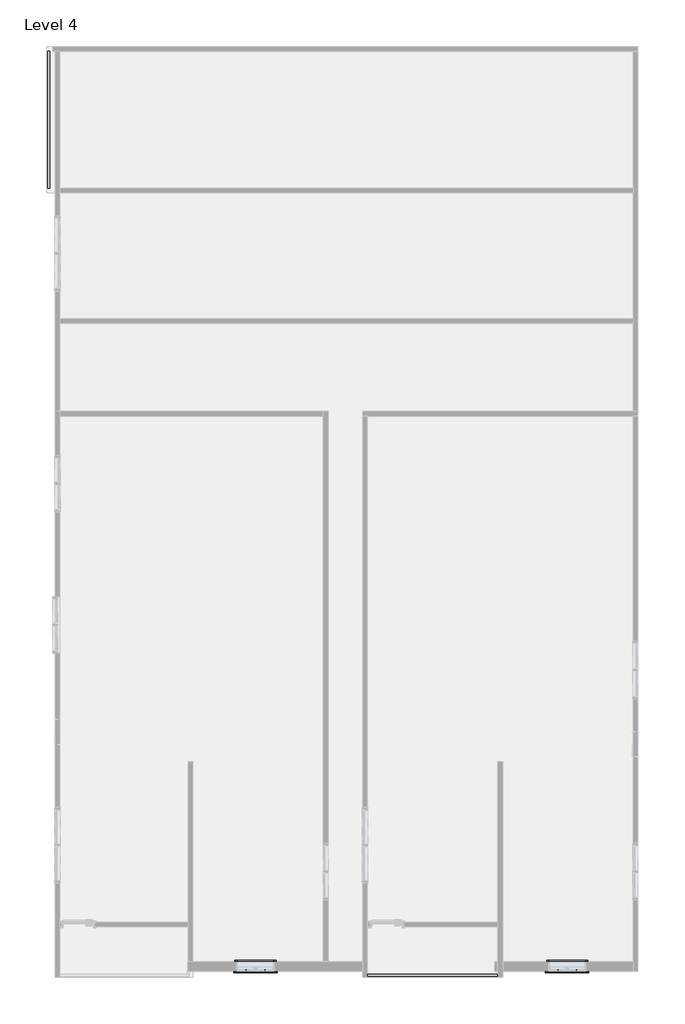
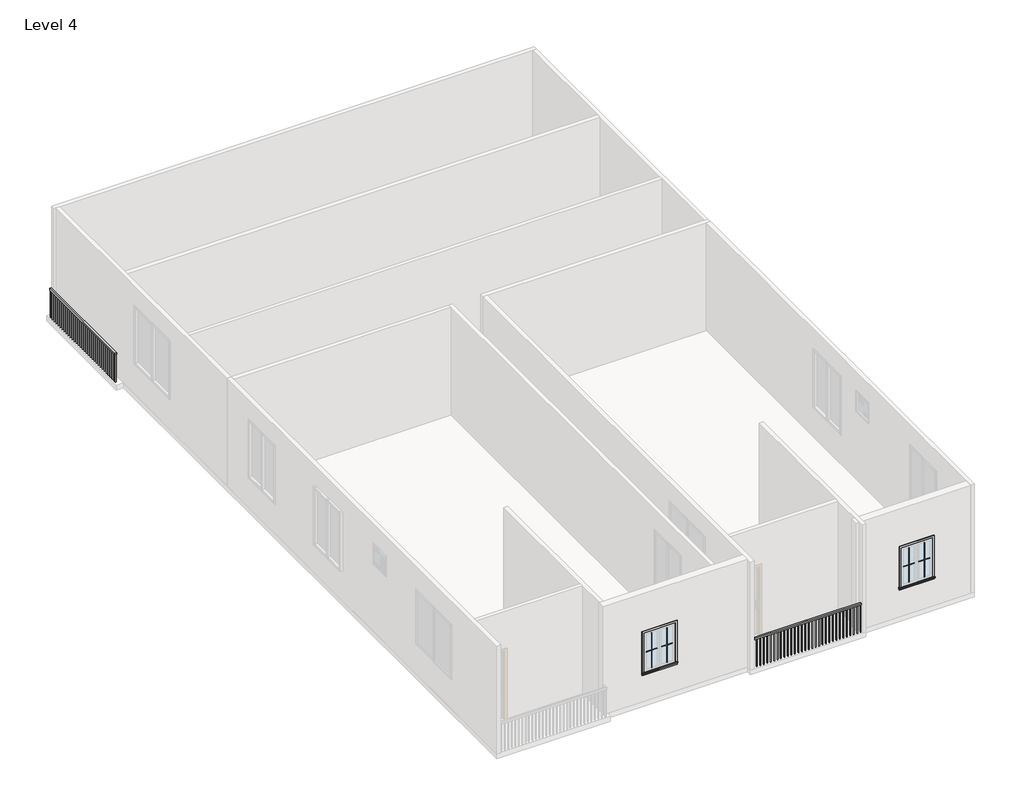
# One storey, part 3 of 3: 8 proxies, 3 railings.
"""IFC4 building model written with IfcOpenShell, lengths in millimetres."""

from ifc_helpers import new_model, si_unit, frame, origin, place, context, project, spatial, polyline, outline, extrude, transform, mapped, element, save
from components import muntin_pattern_2x2_muntin_pattern_2x2_1acec82f, muntin_pattern_2x2_muntin_pattern_2x2_43d02eee, trim_window_exterior_flat_with_sill_e4b28ec3, trim_window_interior_flat_picture_frame_39ff4276

model = new_model("IFC4")

# Units and contexts
model_context = context("Model", 3, world=origin())
ifc_project = project(units=[si_unit("LENGTHUNIT", "METRE", prefix="MILLI")], contexts=[model_context])

# Site, building, storey
site = spatial("IfcSite", under=ifc_project)
building = spatial("IfcBuilding", under=site)
storey = spatial("IfcBuildingStorey", under=building, Name="Level 4", Elevation=10058.4)

# Proxies
placement = place(None, origin())
muntin_pattern_2x2_muntin_pattern_2x2_shape = muntin_pattern_2x2_muntin_pattern_2x2_1acec82f(model_context)
element("IfcBuildingElementProxy", 1, Name="Muntin Pattern_2x2 : Muntin Pattern_2x2", ObjectType="Muntin Pattern_2x2 : Muntin Pattern_2x2", at=placement, inside=storey, context=model_context, shape_type="MappedRepresentation", body=[
    mapped(muntin_pattern_2x2_muntin_pattern_2x2_shape, transform((-3129.6612038, -10576.3529557, 11042.65), x_axis=(-1.0, 0.0, 0.0), y_axis=(0.0, -1.0, 0.0), z_axis=(0.0, 0.0, 1.0))),
])
element("IfcBuildingElementProxy", 2, Name="Muntin Pattern_2x2 : Muntin Pattern_2x2", ObjectType="Muntin Pattern_2x2 : Muntin Pattern_2x2", at=placement, inside=storey, context=model_context, shape_type="MappedRepresentation", body=[
    mapped(muntin_pattern_2x2_muntin_pattern_2x2_shape, transform((4424.1833786, -10576.3529557, 11042.65), x_axis=(-1.0, 0.0, 0.0), y_axis=(0.0, -1.0, 0.0), z_axis=(0.0, 0.0, 1.0))),
])
muntin_pattern_2x2_muntin_pattern_2x2_2_shape = muntin_pattern_2x2_muntin_pattern_2x2_43d02eee(model_context)
element("IfcBuildingElementProxy", 3, Name="Muntin Pattern_2x2 : Muntin Pattern_2x2", ObjectType="Muntin Pattern_2x2 : Muntin Pattern_2x2", at=placement, inside=storey, context=model_context, shape_type="MappedRepresentation", body=[
    mapped(muntin_pattern_2x2_muntin_pattern_2x2_2_shape, transform((-3583.6862038, -10576.3529557, 11042.65), x_axis=(1.0, 0.0, 0.0), y_axis=(0.0, 1.0, 0.0), z_axis=(0.0, 0.0, 1.0))),
])
element("IfcBuildingElementProxy", 4, Name="Muntin Pattern_2x2 : Muntin Pattern_2x2", ObjectType="Muntin Pattern_2x2 : Muntin Pattern_2x2", at=placement, inside=storey, context=model_context, shape_type="MappedRepresentation", body=[
    mapped(muntin_pattern_2x2_muntin_pattern_2x2_2_shape, transform((3970.1583786, -10576.3529557, 11042.65), x_axis=(1.0, 0.0, 0.0), y_axis=(0.0, 1.0, 0.0), z_axis=(0.0, 0.0, 1.0))),
])
trim_window_exterior_flat_with_sill_shape = trim_window_exterior_flat_with_sill_e4b28ec3(model_context)
element("IfcBuildingElementProxy", 5, Name="Trim-Window-Exterior-Flat : with Sill", ObjectType="Trim-Window-Exterior-Flat : with Sill", at=placement, inside=storey, context=model_context, shape_type="MappedRepresentation", body=[
    mapped(trim_window_exterior_flat_with_sill_shape, transform((-3356.6737038, -10585.8779557, 12192.0), x_axis=(1.0, 0.0, 0.0), y_axis=(0.0, 0.0, 1.0), z_axis=(0.0, -1.0, 0.0))),
])
element("IfcBuildingElementProxy", 6, Name="Trim-Window-Exterior-Flat : with Sill", ObjectType="Trim-Window-Exterior-Flat : with Sill", at=placement, inside=storey, context=model_context, shape_type="MappedRepresentation", body=[
    mapped(trim_window_exterior_flat_with_sill_shape, transform((4197.1708786, -10585.8779557, 12192.0), x_axis=(1.0, 0.0, 0.0), y_axis=(0.0, 0.0, 1.0), z_axis=(0.0, -1.0, 0.0))),
])
trim_window_interior_flat_picture_frame_shape = trim_window_interior_flat_picture_frame_39ff4276(model_context)
element("IfcBuildingElementProxy", 7, Name="Trim-Window-Interior-Flat : Picture Frame", ObjectType="Trim-Window-Interior-Flat : Picture Frame", at=placement, inside=storey, context=model_context, shape_type="MappedRepresentation", body=[
    mapped(trim_window_interior_flat_picture_frame_shape, transform((-3356.6737038, -10357.2779557, 12192.0), x_axis=(-1.0, 0.0, 0.0), y_axis=(0.0, 0.0, 1.0), z_axis=(0.0, 1.0, 0.0))),
])
element("IfcBuildingElementProxy", 8, Name="Trim-Window-Interior-Flat : Picture Frame", ObjectType="Trim-Window-Interior-Flat : Picture Frame", at=placement, inside=storey, context=model_context, shape_type="MappedRepresentation", body=[
    mapped(trim_window_interior_flat_picture_frame_shape, transform((4197.1708786, -10357.2779557, 12192.0), x_axis=(-1.0, 0.0, 0.0), y_axis=(0.0, 0.0, 1.0), z_axis=(0.0, 1.0, 0.0))),
])

# Railings
element("IfcRailing", 9, ObjectType="Handrail - Rectangular", at=placement, inside=storey, context=model_context, shape_type="SweptSolid", body=[
    extrude(outline(polyline([(-648.5431282, -10709.8005933), (-648.5431282, -10659.0005933), (2515.990751, -10659.0005933), (2515.990751, -10709.8005933), (-648.5431282, -10709.8005933)])), frame((0.0, 0.0, 10922.0), z_axis=(0.0, 0.0, 1.0), x_axis=(1.0, 0.0, 0.0)), (0.0, 0.0, 1.0), 50.8),
    extrude(outline(polyline([(2491.5318718, -10693.9255933), (2491.5318718, -10674.8755933), (2510.5818718, -10674.8755933), (2510.5818718, -10693.9255933), (2491.5318718, -10693.9255933)])), frame((0.0, 0.0, 10058.4), z_axis=(0.0, 0.0, 1.0), x_axis=(1.0, 0.0, 0.0)), (0.0, 0.0, 1.0), 863.6),
    extrude(outline(polyline([(2389.9318718, -10693.9255933), (2389.9318718, -10674.8755933), (2408.9818718, -10674.8755933), (2408.9818718, -10693.9255933), (2389.9318718, -10693.9255933)])), frame((0.0, 0.0, 10058.4), z_axis=(0.0, 0.0, 1.0), x_axis=(1.0, 0.0, 0.0)), (0.0, 0.0, 1.0), 863.6),
    extrude(outline(polyline([(2288.3318718, -10693.9255933), (2288.3318718, -10674.8755933), (2307.3818718, -10674.8755933), (2307.3818718, -10693.9255933), (2288.3318718, -10693.9255933)])), frame((0.0, 0.0, 10058.4), z_axis=(0.0, 0.0, 1.0), x_axis=(1.0, 0.0, 0.0)), (0.0, 0.0, 1.0), 863.6),
    extrude(outline(polyline([(2186.7318718, -10693.9255933), (2186.7318718, -10674.8755933), (2205.7818718, -10674.8755933), (2205.7818718, -10693.9255933), (2186.7318718, -10693.9255933)])), frame((0.0, 0.0, 10058.4), z_axis=(0.0, 0.0, 1.0), x_axis=(1.0, 0.0, 0.0)), (0.0, 0.0, 1.0), 863.6),
    extrude(outline(polyline([(2085.1318718, -10693.9255933), (2085.1318718, -10674.8755933), (2104.1818718, -10674.8755933), (2104.1818718, -10693.9255933), (2085.1318718, -10693.9255933)])), frame((0.0, 0.0, 10058.4), z_axis=(0.0, 0.0, 1.0), x_axis=(1.0, 0.0, 0.0)), (0.0, 0.0, 1.0), 863.6),
    extrude(outline(polyline([(1983.5318718, -10693.9255933), (1983.5318718, -10674.8755933), (2002.5818718, -10674.8755933), (2002.5818718, -10693.9255933), (1983.5318718, -10693.9255933)])), frame((0.0, 0.0, 10058.4), z_axis=(0.0, 0.0, 1.0), x_axis=(1.0, 0.0, 0.0)), (0.0, 0.0, 1.0), 863.6),
    extrude(outline(polyline([(1881.9318718, -10693.9255933), (1881.9318718, -10674.8755933), (1900.9818718, -10674.8755933), (1900.9818718, -10693.9255933), (1881.9318718, -10693.9255933)])), frame((0.0, 0.0, 10058.4), z_axis=(0.0, 0.0, 1.0), x_axis=(1.0, 0.0, 0.0)), (0.0, 0.0, 1.0), 863.6),
    extrude(outline(polyline([(1780.3318718, -10693.9255933), (1780.3318718, -10674.8755933), (1799.3818718, -10674.8755933), (1799.3818718, -10693.9255933), (1780.3318718, -10693.9255933)])), frame((0.0, 0.0, 10058.4), z_axis=(0.0, 0.0, 1.0), x_axis=(1.0, 0.0, 0.0)), (0.0, 0.0, 1.0), 863.6),
    extrude(outline(polyline([(1678.7318718, -10693.9255933), (1678.7318718, -10674.8755933), (1697.7818718, -10674.8755933), (1697.7818718, -10693.9255933), (1678.7318718, -10693.9255933)])), frame((0.0, 0.0, 10058.4), z_axis=(0.0, 0.0, 1.0), x_axis=(1.0, 0.0, 0.0)), (0.0, 0.0, 1.0), 863.6),
    extrude(outline(polyline([(1577.1318718, -10693.9255933), (1577.1318718, -10674.8755933), (1596.1818718, -10674.8755933), (1596.1818718, -10693.9255933), (1577.1318718, -10693.9255933)])), frame((0.0, 0.0, 10058.4), z_axis=(0.0, 0.0, 1.0), x_axis=(1.0, 0.0, 0.0)), (0.0, 0.0, 1.0), 863.6),
    extrude(outline(polyline([(1475.5318718, -10693.9255933), (1475.5318718, -10674.8755933), (1494.5818718, -10674.8755933), (1494.5818718, -10693.9255933), (1475.5318718, -10693.9255933)])), frame((0.0, 0.0, 10058.4), z_axis=(0.0, 0.0, 1.0), x_axis=(1.0, 0.0, 0.0)), (0.0, 0.0, 1.0), 863.6),
    extrude(outline(polyline([(1373.9318718, -10693.9255933), (1373.9318718, -10674.8755933), (1392.9818718, -10674.8755933), (1392.9818718, -10693.9255933), (1373.9318718, -10693.9255933)])), frame((0.0, 0.0, 10058.4), z_axis=(0.0, 0.0, 1.0), x_axis=(1.0, 0.0, 0.0)), (0.0, 0.0, 1.0), 863.6),
    extrude(outline(polyline([(1272.3318718, -10693.9255933), (1272.3318718, -10674.8755933), (1291.3818718, -10674.8755933), (1291.3818718, -10693.9255933), (1272.3318718, -10693.9255933)])), frame((0.0, 0.0, 10058.4), z_axis=(0.0, 0.0, 1.0), x_axis=(1.0, 0.0, 0.0)), (0.0, 0.0, 1.0), 863.6),
    extrude(outline(polyline([(1170.7318718, -10693.9255933), (1170.7318718, -10674.8755933), (1189.7818718, -10674.8755933), (1189.7818718, -10693.9255933), (1170.7318718, -10693.9255933)])), frame((0.0, 0.0, 10058.4), z_axis=(0.0, 0.0, 1.0), x_axis=(1.0, 0.0, 0.0)), (0.0, 0.0, 1.0), 863.6),
    extrude(outline(polyline([(1069.1318718, -10693.9255933), (1069.1318718, -10674.8755933), (1088.1818718, -10674.8755933), (1088.1818718, -10693.9255933), (1069.1318718, -10693.9255933)])), frame((0.0, 0.0, 10058.4), z_axis=(0.0, 0.0, 1.0), x_axis=(1.0, 0.0, 0.0)), (0.0, 0.0, 1.0), 863.6),
    extrude(outline(polyline([(967.5318718, -10693.9255933), (967.5318718, -10674.8755933), (986.5818718, -10674.8755933), (986.5818718, -10693.9255933), (967.5318718, -10693.9255933)])), frame((0.0, 0.0, 10058.4), z_axis=(0.0, 0.0, 1.0), x_axis=(1.0, 0.0, 0.0)), (0.0, 0.0, 1.0), 863.6),
    extrude(outline(polyline([(865.9318718, -10693.9255933), (865.9318718, -10674.8755933), (884.9818718, -10674.8755933), (884.9818718, -10693.9255933), (865.9318718, -10693.9255933)])), frame((0.0, 0.0, 10058.4), z_axis=(0.0, 0.0, 1.0), x_axis=(1.0, 0.0, 0.0)), (0.0, 0.0, 1.0), 863.6),
    extrude(outline(polyline([(764.3318718, -10693.9255933), (764.3318718, -10674.8755933), (783.3818718, -10674.8755933), (783.3818718, -10693.9255933), (764.3318718, -10693.9255933)])), frame((0.0, 0.0, 10058.4), z_axis=(0.0, 0.0, 1.0), x_axis=(1.0, 0.0, 0.0)), (0.0, 0.0, 1.0), 863.6),
    extrude(outline(polyline([(662.7318718, -10693.9255933), (662.7318718, -10674.8755933), (681.7818718, -10674.8755933), (681.7818718, -10693.9255933), (662.7318718, -10693.9255933)])), frame((0.0, 0.0, 10058.4), z_axis=(0.0, 0.0, 1.0), x_axis=(1.0, 0.0, 0.0)), (0.0, 0.0, 1.0), 863.6),
    extrude(outline(polyline([(561.1318718, -10693.9255933), (561.1318718, -10674.8755933), (580.1818718, -10674.8755933), (580.1818718, -10693.9255933), (561.1318718, -10693.9255933)])), frame((0.0, 0.0, 10058.4), z_axis=(0.0, 0.0, 1.0), x_axis=(1.0, 0.0, 0.0)), (0.0, 0.0, 1.0), 863.6),
    extrude(outline(polyline([(459.5318718, -10693.9255933), (459.5318718, -10674.8755933), (478.5818718, -10674.8755933), (478.5818718, -10693.9255933), (459.5318718, -10693.9255933)])), frame((0.0, 0.0, 10058.4), z_axis=(0.0, 0.0, 1.0), x_axis=(1.0, 0.0, 0.0)), (0.0, 0.0, 1.0), 863.6),
    extrude(outline(polyline([(357.9318718, -10693.9255933), (357.9318718, -10674.8755933), (376.9818718, -10674.8755933), (376.9818718, -10693.9255933), (357.9318718, -10693.9255933)])), frame((0.0, 0.0, 10058.4), z_axis=(0.0, 0.0, 1.0), x_axis=(1.0, 0.0, 0.0)), (0.0, 0.0, 1.0), 863.6),
    extrude(outline(polyline([(256.3318718, -10693.9255933), (256.3318718, -10674.8755933), (275.3818718, -10674.8755933), (275.3818718, -10693.9255933), (256.3318718, -10693.9255933)])), frame((0.0, 0.0, 10058.4), z_axis=(0.0, 0.0, 1.0), x_axis=(1.0, 0.0, 0.0)), (0.0, 0.0, 1.0), 863.6),
    extrude(outline(polyline([(154.7318718, -10693.9255933), (154.7318718, -10674.8755933), (173.7818718, -10674.8755933), (173.7818718, -10693.9255933), (154.7318718, -10693.9255933)])), frame((0.0, 0.0, 10058.4), z_axis=(0.0, 0.0, 1.0), x_axis=(1.0, 0.0, 0.0)), (0.0, 0.0, 1.0), 863.6),
    extrude(outline(polyline([(53.1318718, -10693.9255933), (53.1318718, -10674.8755933), (72.1818718, -10674.8755933), (72.1818718, -10693.9255933), (53.1318718, -10693.9255933)])), frame((0.0, 0.0, 10058.4), z_axis=(0.0, 0.0, 1.0), x_axis=(1.0, 0.0, 0.0)), (0.0, 0.0, 1.0), 863.6),
    extrude(outline(polyline([(-48.4681282, -10693.9255933), (-48.4681282, -10674.8755933), (-29.4181282, -10674.8755933), (-29.4181282, -10693.9255933), (-48.4681282, -10693.9255933)])), frame((0.0, 0.0, 10058.4), z_axis=(0.0, 0.0, 1.0), x_axis=(1.0, 0.0, 0.0)), (0.0, 0.0, 1.0), 863.6),
    extrude(outline(polyline([(-150.0681282, -10693.9255933), (-150.0681282, -10674.8755933), (-131.0181282, -10674.8755933), (-131.0181282, -10693.9255933), (-150.0681282, -10693.9255933)])), frame((0.0, 0.0, 10058.4), z_axis=(0.0, 0.0, 1.0), x_axis=(1.0, 0.0, 0.0)), (0.0, 0.0, 1.0), 863.6),
    extrude(outline(polyline([(-251.6681282, -10693.9255933), (-251.6681282, -10674.8755933), (-232.6181282, -10674.8755933), (-232.6181282, -10693.9255933), (-251.6681282, -10693.9255933)])), frame((0.0, 0.0, 10058.4), z_axis=(0.0, 0.0, 1.0), x_axis=(1.0, 0.0, 0.0)), (0.0, 0.0, 1.0), 863.6),
    extrude(outline(polyline([(-353.2681282, -10693.9255933), (-353.2681282, -10674.8755933), (-334.2181282, -10674.8755933), (-334.2181282, -10693.9255933), (-353.2681282, -10693.9255933)])), frame((0.0, 0.0, 10058.4), z_axis=(0.0, 0.0, 1.0), x_axis=(1.0, 0.0, 0.0)), (0.0, 0.0, 1.0), 863.6),
    extrude(outline(polyline([(-454.8681282, -10693.9255933), (-454.8681282, -10674.8755933), (-435.8181282, -10674.8755933), (-435.8181282, -10693.9255933), (-454.8681282, -10693.9255933)])), frame((0.0, 0.0, 10058.4), z_axis=(0.0, 0.0, 1.0), x_axis=(1.0, 0.0, 0.0)), (0.0, 0.0, 1.0), 863.6),
    extrude(outline(polyline([(-556.4681282, -10693.9255933), (-556.4681282, -10674.8755933), (-537.4181282, -10674.8755933), (-537.4181282, -10693.9255933), (-556.4681282, -10693.9255933)])), frame((0.0, 0.0, 10058.4), z_axis=(0.0, 0.0, 1.0), x_axis=(1.0, 0.0, 0.0)), (0.0, 0.0, 1.0), 863.6),
    extrude(outline(polyline([(2496.940751, -10693.9255933), (2496.940751, -10674.8755933), (2515.990751, -10674.8755933), (2515.990751, -10693.9255933), (2496.940751, -10693.9255933)])), frame((0.0, 0.0, 10058.4), z_axis=(0.0, 0.0, 1.0), x_axis=(1.0, 0.0, 0.0)), (0.0, 0.0, 1.0), 863.6),
    extrude(outline(polyline([(-648.5431282, -10693.9255933), (-648.5431282, -10674.8755933), (-629.4931282, -10674.8755933), (-629.4931282, -10693.9255933), (-648.5431282, -10693.9255933)])), frame((0.0, 0.0, 10058.4), z_axis=(0.0, 0.0, 1.0), x_axis=(1.0, 0.0, 0.0)), (0.0, 0.0, 1.0), 863.6),
])
element("IfcRailing", 10, ObjectType="Handrail - Rectangular", at=placement, inside=storey, context=model_context, shape_type="SweptSolid", body=[
    extrude(outline(polyline([(-8391.7551246, 11703.9189683), (-8340.9551246, 11703.9189683), (-8340.9551246, 8387.4224771), (-8391.7551246, 8387.4224771), (-8391.7551246, 11703.9189683)])), frame((0.0, 0.0, 10922.0), z_axis=(0.0, 0.0, 1.0), x_axis=(1.0, 0.0, 0.0)), (0.0, 0.0, 1.0), 50.8),
    extrude(outline(polyline([(-8375.8801246, 8462.2439683), (-8356.8301246, 8462.2439683), (-8356.8301246, 8443.1939683), (-8375.8801246, 8443.1939683), (-8375.8801246, 8462.2439683)])), frame((0.0, 0.0, 10058.4), z_axis=(0.0, 0.0, 1.0), x_axis=(1.0, 0.0, 0.0)), (0.0, 0.0, 1.0), 863.6),
    extrude(outline(polyline([(-8375.8801246, 8563.8439683), (-8356.8301246, 8563.8439683), (-8356.8301246, 8544.7939683), (-8375.8801246, 8544.7939683), (-8375.8801246, 8563.8439683)])), frame((0.0, 0.0, 10058.4), z_axis=(0.0, 0.0, 1.0), x_axis=(1.0, 0.0, 0.0)), (0.0, 0.0, 1.0), 863.6),
    extrude(outline(polyline([(-8375.8801246, 8665.4439683), (-8356.8301246, 8665.4439683), (-8356.8301246, 8646.3939683), (-8375.8801246, 8646.3939683), (-8375.8801246, 8665.4439683)])), frame((0.0, 0.0, 10058.4), z_axis=(0.0, 0.0, 1.0), x_axis=(1.0, 0.0, 0.0)), (0.0, 0.0, 1.0), 863.6),
    extrude(outline(polyline([(-8375.8801246, 8767.0439683), (-8356.8301246, 8767.0439683), (-8356.8301246, 8747.9939683), (-8375.8801246, 8747.9939683), (-8375.8801246, 8767.0439683)])), frame((0.0, 0.0, 10058.4), z_axis=(0.0, 0.0, 1.0), x_axis=(1.0, 0.0, 0.0)), (0.0, 0.0, 1.0), 863.6),
    extrude(outline(polyline([(-8375.8801246, 8868.6439683), (-8356.8301246, 8868.6439683), (-8356.8301246, 8849.5939683), (-8375.8801246, 8849.5939683), (-8375.8801246, 8868.6439683)])), frame((0.0, 0.0, 10058.4), z_axis=(0.0, 0.0, 1.0), x_axis=(1.0, 0.0, 0.0)), (0.0, 0.0, 1.0), 863.6),
    extrude(outline(polyline([(-8375.8801246, 8970.2439683), (-8356.8301246, 8970.2439683), (-8356.8301246, 8951.1939683), (-8375.8801246, 8951.1939683), (-8375.8801246, 8970.2439683)])), frame((0.0, 0.0, 10058.4), z_axis=(0.0, 0.0, 1.0), x_axis=(1.0, 0.0, 0.0)), (0.0, 0.0, 1.0), 863.6),
    extrude(outline(polyline([(-8375.8801246, 9071.8439683), (-8356.8301246, 9071.8439683), (-8356.8301246, 9052.7939683), (-8375.8801246, 9052.7939683), (-8375.8801246, 9071.8439683)])), frame((0.0, 0.0, 10058.4), z_axis=(0.0, 0.0, 1.0), x_axis=(1.0, 0.0, 0.0)), (0.0, 0.0, 1.0), 863.6),
    extrude(outline(polyline([(-8375.8801246, 9173.4439683), (-8356.8301246, 9173.4439683), (-8356.8301246, 9154.3939683), (-8375.8801246, 9154.3939683), (-8375.8801246, 9173.4439683)])), frame((0.0, 0.0, 10058.4), z_axis=(0.0, 0.0, 1.0), x_axis=(1.0, 0.0, 0.0)), (0.0, 0.0, 1.0), 863.6),
    extrude(outline(polyline([(-8375.8801246, 9275.0439683), (-8356.8301246, 9275.0439683), (-8356.8301246, 9255.9939683), (-8375.8801246, 9255.9939683), (-8375.8801246, 9275.0439683)])), frame((0.0, 0.0, 10058.4), z_axis=(0.0, 0.0, 1.0), x_axis=(1.0, 0.0, 0.0)), (0.0, 0.0, 1.0), 863.6),
    extrude(outline(polyline([(-8375.8801246, 9376.6439683), (-8356.8301246, 9376.6439683), (-8356.8301246, 9357.5939683), (-8375.8801246, 9357.5939683), (-8375.8801246, 9376.6439683)])), frame((0.0, 0.0, 10058.4), z_axis=(0.0, 0.0, 1.0), x_axis=(1.0, 0.0, 0.0)), (0.0, 0.0, 1.0), 863.6),
    extrude(outline(polyline([(-8375.8801246, 9478.2439683), (-8356.8301246, 9478.2439683), (-8356.8301246, 9459.1939683), (-8375.8801246, 9459.1939683), (-8375.8801246, 9478.2439683)])), frame((0.0, 0.0, 10058.4), z_axis=(0.0, 0.0, 1.0), x_axis=(1.0, 0.0, 0.0)), (0.0, 0.0, 1.0), 863.6),
    extrude(outline(polyline([(-8375.8801246, 9579.8439683), (-8356.8301246, 9579.8439683), (-8356.8301246, 9560.7939683), (-8375.8801246, 9560.7939683), (-8375.8801246, 9579.8439683)])), frame((0.0, 0.0, 10058.4), z_axis=(0.0, 0.0, 1.0), x_axis=(1.0, 0.0, 0.0)), (0.0, 0.0, 1.0), 863.6),
    extrude(outline(polyline([(-8375.8801246, 9681.4439683), (-8356.8301246, 9681.4439683), (-8356.8301246, 9662.3939683), (-8375.8801246, 9662.3939683), (-8375.8801246, 9681.4439683)])), frame((0.0, 0.0, 10058.4), z_axis=(0.0, 0.0, 1.0), x_axis=(1.0, 0.0, 0.0)), (0.0, 0.0, 1.0), 863.6),
    extrude(outline(polyline([(-8375.8801246, 9783.0439683), (-8356.8301246, 9783.0439683), (-8356.8301246, 9763.9939683), (-8375.8801246, 9763.9939683), (-8375.8801246, 9783.0439683)])), frame((0.0, 0.0, 10058.4), z_axis=(0.0, 0.0, 1.0), x_axis=(1.0, 0.0, 0.0)), (0.0, 0.0, 1.0), 863.6),
    extrude(outline(polyline([(-8375.8801246, 9884.6439683), (-8356.8301246, 9884.6439683), (-8356.8301246, 9865.5939683), (-8375.8801246, 9865.5939683), (-8375.8801246, 9884.6439683)])), frame((0.0, 0.0, 10058.4), z_axis=(0.0, 0.0, 1.0), x_axis=(1.0, 0.0, 0.0)), (0.0, 0.0, 1.0), 863.6),
    extrude(outline(polyline([(-8375.8801246, 9986.2439683), (-8356.8301246, 9986.2439683), (-8356.8301246, 9967.1939683), (-8375.8801246, 9967.1939683), (-8375.8801246, 9986.2439683)])), frame((0.0, 0.0, 10058.4), z_axis=(0.0, 0.0, 1.0), x_axis=(1.0, 0.0, 0.0)), (0.0, 0.0, 1.0), 863.6),
    extrude(outline(polyline([(-8375.8801246, 10087.8439683), (-8356.8301246, 10087.8439683), (-8356.8301246, 10068.7939683), (-8375.8801246, 10068.7939683), (-8375.8801246, 10087.8439683)])), frame((0.0, 0.0, 10058.4), z_axis=(0.0, 0.0, 1.0), x_axis=(1.0, 0.0, 0.0)), (0.0, 0.0, 1.0), 863.6),
    extrude(outline(polyline([(-8375.8801246, 10189.4439683), (-8356.8301246, 10189.4439683), (-8356.8301246, 10170.3939683), (-8375.8801246, 10170.3939683), (-8375.8801246, 10189.4439683)])), frame((0.0, 0.0, 10058.4), z_axis=(0.0, 0.0, 1.0), x_axis=(1.0, 0.0, 0.0)), (0.0, 0.0, 1.0), 863.6),
    extrude(outline(polyline([(-8375.8801246, 10291.0439683), (-8356.8301246, 10291.0439683), (-8356.8301246, 10271.9939683), (-8375.8801246, 10271.9939683), (-8375.8801246, 10291.0439683)])), frame((0.0, 0.0, 10058.4), z_axis=(0.0, 0.0, 1.0), x_axis=(1.0, 0.0, 0.0)), (0.0, 0.0, 1.0), 863.6),
    extrude(outline(polyline([(-8375.8801246, 10392.6439683), (-8356.8301246, 10392.6439683), (-8356.8301246, 10373.5939683), (-8375.8801246, 10373.5939683), (-8375.8801246, 10392.6439683)])), frame((0.0, 0.0, 10058.4), z_axis=(0.0, 0.0, 1.0), x_axis=(1.0, 0.0, 0.0)), (0.0, 0.0, 1.0), 863.6),
    extrude(outline(polyline([(-8375.8801246, 10494.2439683), (-8356.8301246, 10494.2439683), (-8356.8301246, 10475.1939683), (-8375.8801246, 10475.1939683), (-8375.8801246, 10494.2439683)])), frame((0.0, 0.0, 10058.4), z_axis=(0.0, 0.0, 1.0), x_axis=(1.0, 0.0, 0.0)), (0.0, 0.0, 1.0), 863.6),
    extrude(outline(polyline([(-8375.8801246, 10595.8439683), (-8356.8301246, 10595.8439683), (-8356.8301246, 10576.7939683), (-8375.8801246, 10576.7939683), (-8375.8801246, 10595.8439683)])), frame((0.0, 0.0, 10058.4), z_axis=(0.0, 0.0, 1.0), x_axis=(1.0, 0.0, 0.0)), (0.0, 0.0, 1.0), 863.6),
    extrude(outline(polyline([(-8375.8801246, 10697.4439683), (-8356.8301246, 10697.4439683), (-8356.8301246, 10678.3939683), (-8375.8801246, 10678.3939683), (-8375.8801246, 10697.4439683)])), frame((0.0, 0.0, 10058.4), z_axis=(0.0, 0.0, 1.0), x_axis=(1.0, 0.0, 0.0)), (0.0, 0.0, 1.0), 863.6),
    extrude(outline(polyline([(-8375.8801246, 10799.0439683), (-8356.8301246, 10799.0439683), (-8356.8301246, 10779.9939683), (-8375.8801246, 10779.9939683), (-8375.8801246, 10799.0439683)])), frame((0.0, 0.0, 10058.4), z_axis=(0.0, 0.0, 1.0), x_axis=(1.0, 0.0, 0.0)), (0.0, 0.0, 1.0), 863.6),
    extrude(outline(polyline([(-8375.8801246, 10900.6439683), (-8356.8301246, 10900.6439683), (-8356.8301246, 10881.5939683), (-8375.8801246, 10881.5939683), (-8375.8801246, 10900.6439683)])), frame((0.0, 0.0, 10058.4), z_axis=(0.0, 0.0, 1.0), x_axis=(1.0, 0.0, 0.0)), (0.0, 0.0, 1.0), 863.6),
    extrude(outline(polyline([(-8375.8801246, 11002.2439683), (-8356.8301246, 11002.2439683), (-8356.8301246, 10983.1939683), (-8375.8801246, 10983.1939683), (-8375.8801246, 11002.2439683)])), frame((0.0, 0.0, 10058.4), z_axis=(0.0, 0.0, 1.0), x_axis=(1.0, 0.0, 0.0)), (0.0, 0.0, 1.0), 863.6),
    extrude(outline(polyline([(-8375.8801246, 11103.8439683), (-8356.8301246, 11103.8439683), (-8356.8301246, 11084.7939683), (-8375.8801246, 11084.7939683), (-8375.8801246, 11103.8439683)])), frame((0.0, 0.0, 10058.4), z_axis=(0.0, 0.0, 1.0), x_axis=(1.0, 0.0, 0.0)), (0.0, 0.0, 1.0), 863.6),
    extrude(outline(polyline([(-8375.8801246, 11205.4439683), (-8356.8301246, 11205.4439683), (-8356.8301246, 11186.3939683), (-8375.8801246, 11186.3939683), (-8375.8801246, 11205.4439683)])), frame((0.0, 0.0, 10058.4), z_axis=(0.0, 0.0, 1.0), x_axis=(1.0, 0.0, 0.0)), (0.0, 0.0, 1.0), 863.6),
    extrude(outline(polyline([(-8375.8801246, 11307.0439683), (-8356.8301246, 11307.0439683), (-8356.8301246, 11287.9939683), (-8375.8801246, 11287.9939683), (-8375.8801246, 11307.0439683)])), frame((0.0, 0.0, 10058.4), z_axis=(0.0, 0.0, 1.0), x_axis=(1.0, 0.0, 0.0)), (0.0, 0.0, 1.0), 863.6),
    extrude(outline(polyline([(-8375.8801246, 11408.6439683), (-8356.8301246, 11408.6439683), (-8356.8301246, 11389.5939683), (-8375.8801246, 11389.5939683), (-8375.8801246, 11408.6439683)])), frame((0.0, 0.0, 10058.4), z_axis=(0.0, 0.0, 1.0), x_axis=(1.0, 0.0, 0.0)), (0.0, 0.0, 1.0), 863.6),
    extrude(outline(polyline([(-8375.8801246, 11510.2439683), (-8356.8301246, 11510.2439683), (-8356.8301246, 11491.1939683), (-8375.8801246, 11491.1939683), (-8375.8801246, 11510.2439683)])), frame((0.0, 0.0, 10058.4), z_axis=(0.0, 0.0, 1.0), x_axis=(1.0, 0.0, 0.0)), (0.0, 0.0, 1.0), 863.6),
    extrude(outline(polyline([(-8375.8801246, 11611.8439683), (-8356.8301246, 11611.8439683), (-8356.8301246, 11592.7939683), (-8375.8801246, 11592.7939683), (-8375.8801246, 11611.8439683)])), frame((0.0, 0.0, 10058.4), z_axis=(0.0, 0.0, 1.0), x_axis=(1.0, 0.0, 0.0)), (0.0, 0.0, 1.0), 863.6),
    extrude(outline(polyline([(-8375.8801246, 8406.4724771), (-8356.8301246, 8406.4724771), (-8356.8301246, 8387.4224771), (-8375.8801246, 8387.4224771), (-8375.8801246, 8406.4724771)])), frame((0.0, 0.0, 10058.4), z_axis=(0.0, 0.0, 1.0), x_axis=(1.0, 0.0, 0.0)), (0.0, 0.0, 1.0), 863.6),
    extrude(outline(polyline([(-8375.8801246, 11703.9189683), (-8356.8301246, 11703.9189683), (-8356.8301246, 11684.8689683), (-8375.8801246, 11684.8689683), (-8375.8801246, 11703.9189683)])), frame((0.0, 0.0, 10058.4), z_axis=(0.0, 0.0, 1.0), x_axis=(1.0, 0.0, 0.0)), (0.0, 0.0, 1.0), 863.6),
])
element("IfcRailing", 11, ObjectType="Handrail - Rectangular", at=placement, inside=storey, context=model_context, shape_type="SweptSolid", body=[
    extrude(outline(polyline([(5830.4721078, 11594.1725279), (5881.2721078, 11594.1725279), (5881.2721078, 8505.5262287), (5830.4721078, 8505.5262287), (5830.4721078, 11594.1725279)])), frame((0.0, 0.0, 10922.0), z_axis=(0.0, 0.0, 1.0), x_axis=(1.0, 0.0, 0.0)), (0.0, 0.0, 1.0), 50.8),
    extrude(outline(polyline([(5846.3471078, 8555.6975279), (5865.3971078, 8555.6975279), (5865.3971078, 8536.6475279), (5846.3471078, 8536.6475279), (5846.3471078, 8555.6975279)])), frame((0.0, 0.0, 10058.4), z_axis=(0.0, 0.0, 1.0), x_axis=(1.0, 0.0, 0.0)), (0.0, 0.0, 1.0), 863.6),
    extrude(outline(polyline([(5846.3471078, 8657.2975279), (5865.3971078, 8657.2975279), (5865.3971078, 8638.2475279), (5846.3471078, 8638.2475279), (5846.3471078, 8657.2975279)])), frame((0.0, 0.0, 10058.4), z_axis=(0.0, 0.0, 1.0), x_axis=(1.0, 0.0, 0.0)), (0.0, 0.0, 1.0), 863.6),
    extrude(outline(polyline([(5846.3471078, 8758.8975279), (5865.3971078, 8758.8975279), (5865.3971078, 8739.8475279), (5846.3471078, 8739.8475279), (5846.3471078, 8758.8975279)])), frame((0.0, 0.0, 10058.4), z_axis=(0.0, 0.0, 1.0), x_axis=(1.0, 0.0, 0.0)), (0.0, 0.0, 1.0), 863.6),
    extrude(outline(polyline([(5846.3471078, 8860.4975279), (5865.3971078, 8860.4975279), (5865.3971078, 8841.4475279), (5846.3471078, 8841.4475279), (5846.3471078, 8860.4975279)])), frame((0.0, 0.0, 10058.4), z_axis=(0.0, 0.0, 1.0), x_axis=(1.0, 0.0, 0.0)), (0.0, 0.0, 1.0), 863.6),
    extrude(outline(polyline([(5846.3471078, 8962.0975279), (5865.3971078, 8962.0975279), (5865.3971078, 8943.0475279), (5846.3471078, 8943.0475279), (5846.3471078, 8962.0975279)])), frame((0.0, 0.0, 10058.4), z_axis=(0.0, 0.0, 1.0), x_axis=(1.0, 0.0, 0.0)), (0.0, 0.0, 1.0), 863.6),
    extrude(outline(polyline([(5846.3471078, 9063.6975279), (5865.3971078, 9063.6975279), (5865.3971078, 9044.6475279), (5846.3471078, 9044.6475279), (5846.3471078, 9063.6975279)])), frame((0.0, 0.0, 10058.4), z_axis=(0.0, 0.0, 1.0), x_axis=(1.0, 0.0, 0.0)), (0.0, 0.0, 1.0), 863.6),
    extrude(outline(polyline([(5846.3471078, 9165.2975279), (5865.3971078, 9165.2975279), (5865.3971078, 9146.2475279), (5846.3471078, 9146.2475279), (5846.3471078, 9165.2975279)])), frame((0.0, 0.0, 10058.4), z_axis=(0.0, 0.0, 1.0), x_axis=(1.0, 0.0, 0.0)), (0.0, 0.0, 1.0), 863.6),
    extrude(outline(polyline([(5846.3471078, 9266.8975279), (5865.3971078, 9266.8975279), (5865.3971078, 9247.8475279), (5846.3471078, 9247.8475279), (5846.3471078, 9266.8975279)])), frame((0.0, 0.0, 10058.4), z_axis=(0.0, 0.0, 1.0), x_axis=(1.0, 0.0, 0.0)), (0.0, 0.0, 1.0), 863.6),
    extrude(outline(polyline([(5846.3471078, 9368.4975279), (5865.3971078, 9368.4975279), (5865.3971078, 9349.4475279), (5846.3471078, 9349.4475279), (5846.3471078, 9368.4975279)])), frame((0.0, 0.0, 10058.4), z_axis=(0.0, 0.0, 1.0), x_axis=(1.0, 0.0, 0.0)), (0.0, 0.0, 1.0), 863.6),
    extrude(outline(polyline([(5846.3471078, 9470.0975279), (5865.3971078, 9470.0975279), (5865.3971078, 9451.0475279), (5846.3471078, 9451.0475279), (5846.3471078, 9470.0975279)])), frame((0.0, 0.0, 10058.4), z_axis=(0.0, 0.0, 1.0), x_axis=(1.0, 0.0, 0.0)), (0.0, 0.0, 1.0), 863.6),
    extrude(outline(polyline([(5846.3471078, 9571.6975279), (5865.3971078, 9571.6975279), (5865.3971078, 9552.6475279), (5846.3471078, 9552.6475279), (5846.3471078, 9571.6975279)])), frame((0.0, 0.0, 10058.4), z_axis=(0.0, 0.0, 1.0), x_axis=(1.0, 0.0, 0.0)), (0.0, 0.0, 1.0), 863.6),
    extrude(outline(polyline([(5846.3471078, 9673.2975279), (5865.3971078, 9673.2975279), (5865.3971078, 9654.2475279), (5846.3471078, 9654.2475279), (5846.3471078, 9673.2975279)])), frame((0.0, 0.0, 10058.4), z_axis=(0.0, 0.0, 1.0), x_axis=(1.0, 0.0, 0.0)), (0.0, 0.0, 1.0), 863.6),
    extrude(outline(polyline([(5846.3471078, 9774.8975279), (5865.3971078, 9774.8975279), (5865.3971078, 9755.8475279), (5846.3471078, 9755.8475279), (5846.3471078, 9774.8975279)])), frame((0.0, 0.0, 10058.4), z_axis=(0.0, 0.0, 1.0), x_axis=(1.0, 0.0, 0.0)), (0.0, 0.0, 1.0), 863.6),
    extrude(outline(polyline([(5846.3471078, 9876.4975279), (5865.3971078, 9876.4975279), (5865.3971078, 9857.4475279), (5846.3471078, 9857.4475279), (5846.3471078, 9876.4975279)])), frame((0.0, 0.0, 10058.4), z_axis=(0.0, 0.0, 1.0), x_axis=(1.0, 0.0, 0.0)), (0.0, 0.0, 1.0), 863.6),
    extrude(outline(polyline([(5846.3471078, 9978.0975279), (5865.3971078, 9978.0975279), (5865.3971078, 9959.0475279), (5846.3471078, 9959.0475279), (5846.3471078, 9978.0975279)])), frame((0.0, 0.0, 10058.4), z_axis=(0.0, 0.0, 1.0), x_axis=(1.0, 0.0, 0.0)), (0.0, 0.0, 1.0), 863.6),
    extrude(outline(polyline([(5846.3471078, 10079.6975279), (5865.3971078, 10079.6975279), (5865.3971078, 10060.6475279), (5846.3471078, 10060.6475279), (5846.3471078, 10079.6975279)])), frame((0.0, 0.0, 10058.4), z_axis=(0.0, 0.0, 1.0), x_axis=(1.0, 0.0, 0.0)), (0.0, 0.0, 1.0), 863.6),
    extrude(outline(polyline([(5846.3471078, 10181.2975279), (5865.3971078, 10181.2975279), (5865.3971078, 10162.2475279), (5846.3471078, 10162.2475279), (5846.3471078, 10181.2975279)])), frame((0.0, 0.0, 10058.4), z_axis=(0.0, 0.0, 1.0), x_axis=(1.0, 0.0, 0.0)), (0.0, 0.0, 1.0), 863.6),
    extrude(outline(polyline([(5846.3471078, 10282.8975279), (5865.3971078, 10282.8975279), (5865.3971078, 10263.8475279), (5846.3471078, 10263.8475279), (5846.3471078, 10282.8975279)])), frame((0.0, 0.0, 10058.4), z_axis=(0.0, 0.0, 1.0), x_axis=(1.0, 0.0, 0.0)), (0.0, 0.0, 1.0), 863.6),
    extrude(outline(polyline([(5846.3471078, 10384.4975279), (5865.3971078, 10384.4975279), (5865.3971078, 10365.4475279), (5846.3471078, 10365.4475279), (5846.3471078, 10384.4975279)])), frame((0.0, 0.0, 10058.4), z_axis=(0.0, 0.0, 1.0), x_axis=(1.0, 0.0, 0.0)), (0.0, 0.0, 1.0), 863.6),
    extrude(outline(polyline([(5846.3471078, 10486.0975279), (5865.3971078, 10486.0975279), (5865.3971078, 10467.0475279), (5846.3471078, 10467.0475279), (5846.3471078, 10486.0975279)])), frame((0.0, 0.0, 10058.4), z_axis=(0.0, 0.0, 1.0), x_axis=(1.0, 0.0, 0.0)), (0.0, 0.0, 1.0), 863.6),
    extrude(outline(polyline([(5846.3471078, 10587.6975279), (5865.3971078, 10587.6975279), (5865.3971078, 10568.6475279), (5846.3471078, 10568.6475279), (5846.3471078, 10587.6975279)])), frame((0.0, 0.0, 10058.4), z_axis=(0.0, 0.0, 1.0), x_axis=(1.0, 0.0, 0.0)), (0.0, 0.0, 1.0), 863.6),
    extrude(outline(polyline([(5846.3471078, 10689.2975279), (5865.3971078, 10689.2975279), (5865.3971078, 10670.2475279), (5846.3471078, 10670.2475279), (5846.3471078, 10689.2975279)])), frame((0.0, 0.0, 10058.4), z_axis=(0.0, 0.0, 1.0), x_axis=(1.0, 0.0, 0.0)), (0.0, 0.0, 1.0), 863.6),
    extrude(outline(polyline([(5846.3471078, 10790.8975279), (5865.3971078, 10790.8975279), (5865.3971078, 10771.8475279), (5846.3471078, 10771.8475279), (5846.3471078, 10790.8975279)])), frame((0.0, 0.0, 10058.4), z_axis=(0.0, 0.0, 1.0), x_axis=(1.0, 0.0, 0.0)), (0.0, 0.0, 1.0), 863.6),
    extrude(outline(polyline([(5846.3471078, 10892.4975279), (5865.3971078, 10892.4975279), (5865.3971078, 10873.4475279), (5846.3471078, 10873.4475279), (5846.3471078, 10892.4975279)])), frame((0.0, 0.0, 10058.4), z_axis=(0.0, 0.0, 1.0), x_axis=(1.0, 0.0, 0.0)), (0.0, 0.0, 1.0), 863.6),
    extrude(outline(polyline([(5846.3471078, 10994.0975279), (5865.3971078, 10994.0975279), (5865.3971078, 10975.0475279), (5846.3471078, 10975.0475279), (5846.3471078, 10994.0975279)])), frame((0.0, 0.0, 10058.4), z_axis=(0.0, 0.0, 1.0), x_axis=(1.0, 0.0, 0.0)), (0.0, 0.0, 1.0), 863.6),
    extrude(outline(polyline([(5846.3471078, 11095.6975279), (5865.3971078, 11095.6975279), (5865.3971078, 11076.6475279), (5846.3471078, 11076.6475279), (5846.3471078, 11095.6975279)])), frame((0.0, 0.0, 10058.4), z_axis=(0.0, 0.0, 1.0), x_axis=(1.0, 0.0, 0.0)), (0.0, 0.0, 1.0), 863.6),
    extrude(outline(polyline([(5846.3471078, 11197.2975279), (5865.3971078, 11197.2975279), (5865.3971078, 11178.2475279), (5846.3471078, 11178.2475279), (5846.3471078, 11197.2975279)])), frame((0.0, 0.0, 10058.4), z_axis=(0.0, 0.0, 1.0), x_axis=(1.0, 0.0, 0.0)), (0.0, 0.0, 1.0), 863.6),
    extrude(outline(polyline([(5846.3471078, 11298.8975279), (5865.3971078, 11298.8975279), (5865.3971078, 11279.8475279), (5846.3471078, 11279.8475279), (5846.3471078, 11298.8975279)])), frame((0.0, 0.0, 10058.4), z_axis=(0.0, 0.0, 1.0), x_axis=(1.0, 0.0, 0.0)), (0.0, 0.0, 1.0), 863.6),
    extrude(outline(polyline([(5846.3471078, 11400.4975279), (5865.3971078, 11400.4975279), (5865.3971078, 11381.4475279), (5846.3471078, 11381.4475279), (5846.3471078, 11400.4975279)])), frame((0.0, 0.0, 10058.4), z_axis=(0.0, 0.0, 1.0), x_axis=(1.0, 0.0, 0.0)), (0.0, 0.0, 1.0), 863.6),
    extrude(outline(polyline([(5846.3471078, 11502.0975279), (5865.3971078, 11502.0975279), (5865.3971078, 11483.0475279), (5846.3471078, 11483.0475279), (5846.3471078, 11502.0975279)])), frame((0.0, 0.0, 10058.4), z_axis=(0.0, 0.0, 1.0), x_axis=(1.0, 0.0, 0.0)), (0.0, 0.0, 1.0), 863.6),
    extrude(outline(polyline([(5846.3471078, 8524.5762287), (5865.3971078, 8524.5762287), (5865.3971078, 8505.5262287), (5846.3471078, 8505.5262287), (5846.3471078, 8524.5762287)])), frame((0.0, 0.0, 10058.4), z_axis=(0.0, 0.0, 1.0), x_axis=(1.0, 0.0, 0.0)), (0.0, 0.0, 1.0), 863.6),
    extrude(outline(polyline([(5846.3471078, 11594.1725279), (5865.3971078, 11594.1725279), (5865.3971078, 11575.1225279), (5846.3471078, 11575.1225279), (5846.3471078, 11594.1725279)])), frame((0.0, 0.0, 10058.4), z_axis=(0.0, 0.0, 1.0), x_axis=(1.0, 0.0, 0.0)), (0.0, 0.0, 1.0), 863.6),
])

save(model, "model.ifc")

# Revit data of these elements
# Type "Muntin Pattern_2x2 : Muntin Pattern_2x2"
#   Width [instance default] = 4' - 0"
#   Thickness = 0' - 0 1/2"
#   Height [instance default] = 4' - 0"
#   Distance = 0' - 0 3/4"
#   Interior Material [instance default] = none
#   Exterior Material [instance default] = none
#   Default Elevation = 0
# Type "Trim-Window-Exterior-Flat : with Sill"
#   Trim Width = 0' - 2 1/4"
#   Trim Thickness_Picture Frame = 0' - 1 1/4"
#   Trim Thickness_with Sill = 0' - 0 3/4"
#   Sill Thickness = 0' - 1 1/4"
#   Opening Width [instance default] = 2' - 0"
#   Opening Height [instance default] = 3' - 0"
#   Default Elevation = 4' - 0"
#   Sill = yes
#   Picture Frame = no
#   Trim Material [instance default] = none
# Type "Trim-Window-Interior-Flat : Picture Frame"
#   Trim Thickness_Picture Frame = 0' - 1 1/4"
#   Trim Width = 0' - 2 1/4"
#   Trim Thickness_with Sill = 0' - 0 3/4"
#   Sill Thickness = 0' - 1 1/4"
#   Opening Width [instance default] = 2' - 0"
#   Opening Height [instance default] = 3' - 0"
#   Default Elevation = 4' - 0"
#   Sill = no
#   Picture Frame = yes
#   Trim Material [instance default] = none
# Type "Handrail - Rectangular"
#   Assembly Code = "C2010400"
#   built-in parameter 1008612 = 0.0416667 (stored number, unit not read)
#   built-in parameter 1008611 = 0.0416667 (stored number, unit not read)
#   built-in parameter 1008609 = 0.333333 (stored number, unit not read)
#   built-in parameter 1008604 = 0.166667 (stored number, unit not read)
#   built-in parameter 1008603 = 0.166667 (stored number, unit not read)
#   Railing Height = 3' - 0"
#   built-in parameter 1008630 = 2
#   built-in parameter 1008610 = 2
#   built-in parameter 1008618 = Baluster - Square : 3/4"
# Elements 1, 2, 3, 4 (IfcBuildingElementProxy, "Muntin Pattern_2x2 : Muntin Pattern_2x2")
#   Width = 1' - 0 5/8"
#   Height = 3' - 6 1/2"
#   Interior Material = Wood - Stained
#   Exterior Material = Clad - White
#   Phase Created = New Construction
#   Materials on its faces: "Clad - White", "Wood - Stained"
# Elements 5, 6 (IfcBuildingElementProxy, "Trim-Window-Exterior-Flat : with Sill")
#   Opening Width = 3' - 0"
#   Opening Height = 4' - 0"
#   Trim Material = Clad - White
#   Phase Created = New Construction
#   Materials on its faces: "Clad - White"
# Elements 7, 8 (IfcBuildingElementProxy, "Trim-Window-Interior-Flat : Picture Frame")
#   Opening Width = 3' - 0"
#   Opening Height = 4' - 0"
#   Trim Material = Wood - Stained
#   Phase Created = New Construction
#   Materials on its faces: "Wood - Stained"
# Elements 9, 10, 11 (IfcRailing, "Handrail - Rectangular")
#   Phase Created = New Construction
# Materials
#   "Clad - White": class "Wood", colour RGB 242 242 238, transparency 0, Cost = 0
#   "Wood - Stained": class "Wood", colour RGB 224 178 126, transparency 0, Cost = 0
